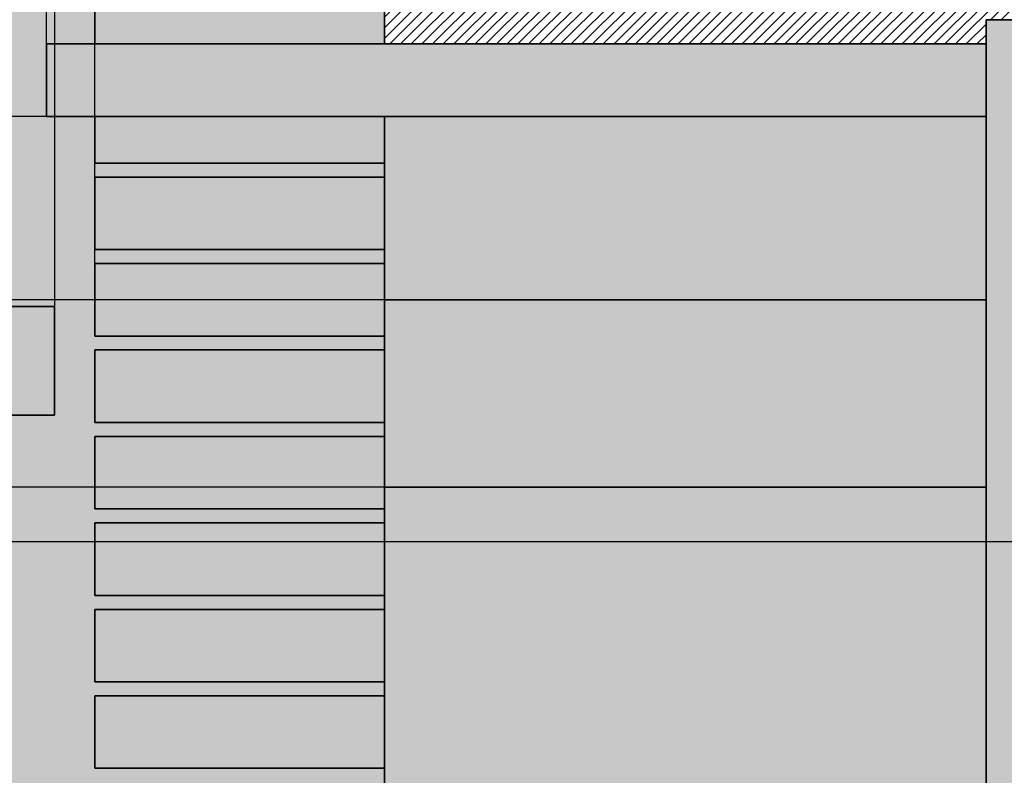
# Model space of a CAD drawing. Units: inches. Extents: x 126 to 726, y 86 to 888.
# Tile 10 of 13: x 426 to 589, y 486 to 611. Entities that reach past the tile are written whole.
import ezdxf

# ---------------------------------------------------------------- set-up
doc = ezdxf.new("R2010")
doc.units = ezdxf.units.IN
doc.header["$MEASUREMENT"] = 0
for name, color, linetype, lineweight in [('A-ANNO-DIMS', 2, 'Continuous', 18), ('A-ELEV', 7, 'Continuous', 35), ('A-ELEV-PATT', 8, 'Continuous', 13)]:
    doc.layers.add(name, color=color, linetype=linetype, lineweight=lineweight)
doc.styles.get("Standard").update_dxf_attribs({"font": 'arial.ttf'})
doc.dimstyles.get("Standard").update_dxf_attribs({"dimtxt": 6, "dimasz": 3, "dimexe": 0.18, "dimexo": 0.0625, "dimgap": 0.09, "dimtad": 0, "dimtih": 1, "dimtoh": 1, "dimdec": 0, "dimzin": 0, "dimdsep": 46, "dimlunit": 3, "dimtxsty": 'Standard', "dimcen": 0.09, "dimadec": 0, "dimazin": 0, "dimtfac": 1, "dimtdec": 0, "dimtofl": 0, "dimtmove": 0, "dimatfit": 3, "dimfxl": 1, "dimtolj": 1, "dimtzin": 0, "dimarcsym": 0})

# ---------------------------------------------------------------- blocks, each defined once
blk = doc.blocks.new('FACADE-STRIP')
for p, q in [((0, 0), (0, 12)), ((0, 12), (48, 12)), ((0, 0), (48, 0))]:
    blk.add_line(p, q)
blk = doc.blocks.new('*D13')
at = {"layer": 'A-ANNO-DIMS', "color": 0, "lineweight": -2, "transparency": 16777216}
for p, q in [((665.97, 642.98), (665.97, 90.21)), ((185.97, 126.98), (185.97, 90.21)), ((188.97, 90.39), (419.15, 90.39)), ((662.97, 90.39), (432.8, 90.39))]:
    blk.add_line(p, q, dxfattribs=at)
at = {"layer": 'A-ANNO-DIMS', "color": 0, "transparency": 16777216}
for points in [[(188.97, 90.89), (188.97, 89.89), (185.97, 90.39)], [(662.97, 90.89), (662.97, 89.89), (665.97, 90.39)]]:
    blk.add_solid(points, dxfattribs=at)
at = {"layer": 'Defpoints', "color": 0, "transparency": 16777216}
for p in [(665.97, 643.04), (185.97, 127.04), (665.97, 90.39)]:
    blk.add_point(p, dxfattribs=at)
at = {"layer": 'A-ANNO-DIMS', "color": 0, "transparency": 16777216, "insert": (425.97, 90.39), "char_height": 6, "attachment_point": 5}
blk.add_mtext('\\A1;480', dxfattribs=at)
blk = doc.blocks.new('*D21')
at = {"layer": 'A-ANNO-DIMS', "color": 0, "lineweight": -2, "transparency": 16777216}
for p, q in [((431.28, 563.58), (149.14, 563.58)), ((149.32, 560.58), (149.32, 557.74)), ((149.32, 548.58), (149.32, 551.43)), ((233.91, 545.58), (149.14, 545.58))]:
    blk.add_line(p, q, dxfattribs=at)
at = {"layer": 'A-ANNO-DIMS', "color": 0, "transparency": 16777216}
for points in [[(148.82, 560.58), (149.82, 560.58), (149.32, 563.58)], [(148.82, 548.58), (149.82, 548.58), (149.32, 545.58)]]:
    blk.add_solid(points, dxfattribs=at)
at = {"layer": 'Defpoints', "color": 0, "transparency": 16777216}
for p in [(149.32, 563.58), (431.34, 563.58), (233.97, 545.58)]:
    blk.add_point(p, dxfattribs=at)
at = {"layer": 'A-ANNO-DIMS', "color": 0, "transparency": 16777216, "insert": (149.32, 554.58), "char_height": 6, "attachment_point": 5}
blk.add_mtext('\\A1;18', dxfattribs=at)
blk = doc.blocks.new('*D22')
at = {"layer": 'A-ANNO-DIMS', "color": 0, "lineweight": -2, "transparency": 16777216}
for p, q in [((185.91, 847.04), (149.14, 847.04)), ((149.32, 844.04), (149.32, 708.47)), ((149.32, 566.58), (149.32, 702.16)), ((431.28, 563.58), (149.14, 563.58))]:
    blk.add_line(p, q, dxfattribs=at)
at = {"layer": 'A-ANNO-DIMS', "color": 0, "transparency": 16777216}
for points in [[(148.82, 844.04), (149.82, 844.04), (149.32, 847.04)], [(148.82, 566.58), (149.82, 566.58), (149.32, 563.58)]]:
    blk.add_solid(points, dxfattribs=at)
at = {"layer": 'Defpoints', "color": 0, "transparency": 16777216}
for p in [(149.32, 847.04), (185.97, 847.04), (431.34, 563.58)]:
    blk.add_point(p, dxfattribs=at)
at = {"layer": 'A-ANNO-DIMS', "color": 0, "transparency": 16777216, "insert": (149.32, 705.31), "char_height": 6, "attachment_point": 5}
blk.add_mtext('\\A1;283.46', dxfattribs=at)
blk = doc.blocks.new('*D34')
at = {"layer": 'A-ANNO-DIMS', "color": 0, "lineweight": -2, "transparency": 16777216}
for p, q in [((362.73, 524.68), (702.8, 524.68)), ((702.62, 521.68), (702.62, 482.84)), ((702.62, 437.68), (702.62, 476.53)), ((362.73, 434.68), (702.8, 434.68))]:
    blk.add_line(p, q, dxfattribs=at)
at = {"layer": 'A-ANNO-DIMS', "color": 0, "transparency": 16777216}
for points in [[(702.12, 521.68), (703.12, 521.68), (702.62, 524.68)], [(702.12, 437.68), (703.12, 437.68), (702.62, 434.68)]]:
    blk.add_solid(points, dxfattribs=at)
at = {"layer": 'Defpoints', "color": 0, "transparency": 16777216}
for p in [(362.67, 524.68), (702.62, 524.68), (362.67, 434.68)]:
    blk.add_point(p, dxfattribs=at)
at = {"layer": 'A-ANNO-DIMS', "color": 0, "transparency": 16777216, "insert": (702.62, 479.68), "char_height": 6, "attachment_point": 5}
blk.add_mtext('\\A1;90', dxfattribs=at)
blk = doc.blocks.new('*D41')
at = {"layer": 'A-ANNO-DIMS', "color": 0, "lineweight": -2, "transparency": 16777216}
for p, q in [((429.97, 607.1), (429.97, 883.87)), ((432.97, 883.69), (541.21, 883.69)), ((662.97, 883.69), (554.74, 883.69)), ((665.97, 607.1), (665.97, 883.87))]:
    blk.add_line(p, q, dxfattribs=at)
at = {"layer": 'A-ANNO-DIMS', "color": 0, "transparency": 16777216}
for points in [[(432.97, 884.19), (432.97, 883.19), (429.97, 883.69)], [(662.97, 884.19), (662.97, 883.19), (665.97, 883.69)]]:
    blk.add_solid(points, dxfattribs=at)
at = {"layer": 'Defpoints', "color": 0, "transparency": 16777216}
for p in [(665.97, 883.69), (429.97, 607.04), (665.97, 607.04)]:
    blk.add_point(p, dxfattribs=at)
at = {"layer": 'A-ANNO-DIMS', "color": 0, "transparency": 16777216, "insert": (547.97, 883.69), "char_height": 6, "attachment_point": 5}
blk.add_mtext('\\A1;236', dxfattribs=at)
blk = doc.blocks.new('*D43')
at = {"layer": 'A-ANNO-DIMS', "color": 0, "lineweight": -2, "transparency": 16777216}
for p, q in [((429.97, 595.1), (429.97, 883.87)), ((432.97, 883.69), (434.97, 883.69)), ((437.97, 585.06), (437.97, 883.87)), ((437.97, 883.69), (440.97, 883.69))]:
    blk.add_line(p, q, dxfattribs=at)
at = {"layer": 'A-ANNO-DIMS', "color": 0, "transparency": 16777216}
for points in [[(432.97, 884.19), (432.97, 883.19), (429.97, 883.69)], [(434.97, 884.19), (434.97, 883.19), (437.97, 883.69)]]:
    blk.add_solid(points, dxfattribs=at)
at = {"layer": 'Defpoints', "color": 0, "transparency": 16777216}
for p in [(437.97, 883.69), (429.97, 595.04), (437.97, 585)]:
    blk.add_point(p, dxfattribs=at)
at = {"layer": 'A-ANNO-DIMS', "color": 0, "transparency": 16777216, "insert": (443.04, 883.69), "char_height": 6, "attachment_point": 5}
blk.add_mtext('\\A1;8', dxfattribs=at)
blk = doc.blocks.new('*D44')
at = {"layer": 'A-ANNO-DIMS', "color": 0, "lineweight": -2, "transparency": 16777216}
for p, q in [((431.34, 563.65), (431.34, 883.87)), ((434.34, 883.69), (434.97, 883.69)), ((437.97, 570.75), (437.97, 883.87)), ((437.97, 883.69), (440.97, 883.69))]:
    blk.add_line(p, q, dxfattribs=at)
at = {"layer": 'A-ANNO-DIMS', "color": 0, "transparency": 16777216}
for points in [[(434.34, 884.19), (434.34, 883.19), (431.34, 883.69)], [(434.97, 884.19), (434.97, 883.19), (437.97, 883.69)]]:
    blk.add_solid(points, dxfattribs=at)
at = {"layer": 'Defpoints', "color": 0, "transparency": 16777216}
for p in [(437.97, 883.69), (437.97, 570.69), (431.34, 563.58)]:
    blk.add_point(p, dxfattribs=at)
at = {"layer": 'A-ANNO-DIMS', "color": 0, "transparency": 16777216, "insert": (451.2, 883.69), "char_height": 6, "attachment_point": 5}
blk.add_mtext('\\A1;6.636', dxfattribs=at)
blk = doc.blocks.new('*D58')
at = {"layer": 'A-ANNO-DIMS', "color": 0, "lineweight": -2, "transparency": 16777216}
for p, q in [((485.91, 533.68), (149.14, 533.68)), ((149.32, 530.68), (149.32, 453.52)), ((149.32, 370.04), (149.32, 447.21)), ((485.91, 367.04), (149.14, 367.04))]:
    blk.add_line(p, q, dxfattribs=at)
at = {"layer": 'A-ANNO-DIMS', "color": 0, "transparency": 16777216}
for points in [[(148.82, 530.68), (149.82, 530.68), (149.32, 533.68)], [(148.82, 370.04), (149.82, 370.04), (149.32, 367.04)]]:
    blk.add_solid(points, dxfattribs=at)
at = {"layer": 'Defpoints', "color": 0, "transparency": 16777216}
for p in [(149.32, 533.68), (485.97, 533.68), (485.97, 367.04)]:
    blk.add_point(p, dxfattribs=at)
at = {"layer": 'A-ANNO-DIMS', "color": 0, "transparency": 16777216, "insert": (149.32, 450.36), "char_height": 6, "attachment_point": 5}
blk.add_mtext('\\A1;166.64', dxfattribs=at)
blk = doc.blocks.new('*D59')
at = {"layer": 'A-ANNO-DIMS', "color": 0, "lineweight": -2, "transparency": 16777216}
for p, q in [((485.91, 564.68), (149.14, 564.68)), ((149.32, 561.68), (149.32, 552.34)), ((149.32, 536.68), (149.32, 546.03)), ((485.91, 533.68), (149.14, 533.68))]:
    blk.add_line(p, q, dxfattribs=at)
at = {"layer": 'A-ANNO-DIMS', "color": 0, "transparency": 16777216}
for points in [[(148.82, 561.68), (149.82, 561.68), (149.32, 564.68)], [(148.82, 536.68), (149.82, 536.68), (149.32, 533.68)]]:
    blk.add_solid(points, dxfattribs=at)
at = {"layer": 'Defpoints', "color": 0, "transparency": 16777216}
for p in [(149.32, 564.68), (485.97, 564.68), (485.97, 533.68)]:
    blk.add_point(p, dxfattribs=at)
at = {"layer": 'A-ANNO-DIMS', "color": 0, "transparency": 16777216, "insert": (149.32, 549.18), "char_height": 6, "attachment_point": 5}
blk.add_mtext('\\A1;31', dxfattribs=at)
blk = doc.blocks.new('*D60')
at = {"layer": 'A-ANNO-DIMS', "color": 0, "lineweight": -2, "transparency": 16777216}
for p, q in [((485.91, 595.04), (149.14, 595.04)), ((149.32, 592.04), (149.32, 583.02)), ((149.32, 567.68), (149.32, 576.71)), ((485.91, 564.68), (149.14, 564.68))]:
    blk.add_line(p, q, dxfattribs=at)
at = {"layer": 'A-ANNO-DIMS', "color": 0, "transparency": 16777216}
for points in [[(148.82, 592.04), (149.82, 592.04), (149.32, 595.04)], [(148.82, 567.68), (149.82, 567.68), (149.32, 564.68)]]:
    blk.add_solid(points, dxfattribs=at)
at = {"layer": 'Defpoints', "color": 0, "transparency": 16777216}
for p in [(149.32, 595.04), (485.97, 595.04), (485.97, 564.68)]:
    blk.add_point(p, dxfattribs=at)
at = {"layer": 'A-ANNO-DIMS', "color": 0, "transparency": 16777216, "insert": (149.32, 579.86), "char_height": 6, "attachment_point": 5}
blk.add_mtext('\\A1;30.36', dxfattribs=at)

msp = doc.modelspace()

# ---------------------------------------------------------------- hatches: boundary and pattern name
at = {"layer": 'A-ELEV-PATT'}
h = msp.add_hatch(color=256, dxfattribs=at)
h.dxf.hatch_style = 1
h.paths.add_polyline_path([(233.9749, 545.5846), (431.3386, 545.5846), (431.3386, 563.5846), (185.9749, 563.5846), (185.9749, 395.5846), (431.3386, 395.5846), (431.3386, 413.5846), (233.9749, 413.5846)])
h.paths.add_polyline_path([(233.9749, 835.0424), (485.9749, 835.0424), (605.9749, 835.0424), (605.9749, 847.0424), (485.9749, 847.0424), (185.9749, 847.0424), (185.9749, 606.5846), (233.9749, 606.5846)])
h.paths.add_polyline_path([(233.9749, 597.5846), (185.9749, 597.5846), (185.9749, 585.5846), (233.9749, 585.5846)])
h.paths.add_polyline_path([(233.9749, 580.5846), (185.9749, 580.5846), (185.9749, 568.5846), (233.9749, 568.5846)])
h = msp.add_hatch(color=256, dxfattribs=at)
h.dxf.hatch_style = 1
h.paths.add_polyline_path([(437.9749, 499.1312), (485.9749, 499.1312), (485.9749, 501.4423), (437.9749, 501.4423), (437.9749, 513.4423), (485.9749, 513.4423), (485.9749, 515.7534), (437.9749, 515.7534), (437.9749, 527.7534), (485.9749, 527.7534), (485.9749, 530.0646), (437.9749, 530.0646), (437.9749, 542.0646), (485.9749, 542.0646), (485.9749, 544.3757), (437.9749, 544.3757), (437.9749, 556.3757), (485.9749, 556.3757), (485.9749, 558.6868), (437.9749, 558.6868), (437.9749, 570.6868), (485.9749, 570.6868), (485.9749, 572.9979), (437.9749, 572.9979), (437.9749, 584.9979), (485.9749, 584.9979), (485.9749, 587.309), (437.9749, 587.309), (437.9749, 595.0424), (429.9749, 595.0424), (429.9749, 607.0424), (437.9749, 607.0424), (437.9749, 615.9312), (437.9749, 630.2423), (437.9749, 642.2423), (485.9749, 642.2423), (485.9749, 644.5534), (437.9749, 644.5534), (437.9749, 656.5534), (485.9749, 656.5534), (485.9749, 658.8645), (437.9749, 658.8645), (437.9749, 670.8645), (485.9749, 670.8645), (485.9749, 673.1757), (437.9749, 673.1757), (437.9749, 685.1757), (485.9749, 685.1757), (485.9749, 687.4868), (437.9749, 687.4868), (437.9749, 699.4868), (485.9749, 699.4868), (485.9749, 701.7979), (437.9749, 701.7979), (437.9749, 713.7979), (485.9749, 713.7979), (485.9749, 716.109), (437.9749, 716.109), (437.9749, 728.109), (485.9749, 728.109), (485.9749, 730.4201), (437.9749, 730.4201), (437.9749, 742.4201), (485.9749, 742.4201), (485.9749, 744.7312), (437.9749, 744.7312), (437.9749, 756.7312), (485.9749, 756.7312), (485.9749, 759.0423), (437.9749, 759.0423), (437.9749, 771.0423), (485.9749, 771.0423), (485.9749, 773.3534), (437.9749, 773.3534), (437.9749, 785.3534), (485.9749, 785.3534), (485.9749, 787.6645), (437.9749, 787.6645), (437.9749, 799.6645), (485.9749, 799.6645), (485.9749, 801.9756), (437.9749, 801.9756), (437.9749, 811.2868), (485.9749, 811.2868), (485.9749, 813.9756), (437.9749, 813.9756), (437.9749, 825.9756), (485.9749, 825.9756), (485.9749, 835.0424), (233.9749, 835.0424), (233.9749, 606.5846), (185.9749, 606.5846), (185.9749, 597.5846), (233.9749, 597.5846), (233.9749, 585.5846), (185.9749, 585.5846), (185.9749, 580.5846), (233.9749, 580.5846), (233.9749, 568.5846), (185.9749, 568.5846), (185.9749, 563.5846), (431.3386, 563.5846), (431.3386, 545.5846), (233.9749, 545.5846), (233.9749, 413.5846), (431.3386, 413.5846), (431.3386, 395.5846), (185.9749, 395.5846), (185.9749, 386.5846), (233.9749, 386.5846), (233.9749, 374.5846), (185.9749, 374.5846), (185.9749, 369.5846), (233.9749, 369.5846), (233.9749, 357.5846), (185.9749, 357.5846), (185.9749, 352.5846), (233.9749, 352.5846), (233.9749, 340.5846), (185.9749, 340.5846), (185.9749, 331.5846), (233.9749, 331.5846), (233.9749, 127.0424), (485.9749, 127.0424), (485.9749, 129.3535), (437.9749, 129.3535), (437.9749, 141.3535), (485.9749, 141.3535), (485.9749, 143.6646), (437.9749, 143.6646), (437.9749, 155.6646), (485.9749, 155.6646), (485.9749, 157.9757), (437.9749, 157.9757), (437.9749, 169.9757), (485.9749, 169.9757), (485.9749, 172.2868), (437.9749, 172.2868), (437.9749, 184.2868), (485.9749, 184.2868), (485.9749, 186.5979), (437.9749, 186.5979), (437.9749, 198.5979), (485.9749, 198.5979), (485.9749, 200.909), (437.9749, 200.909), (437.9749, 212.909), (485.9749, 212.909), (485.9749, 215.2201), (437.9749, 215.2201), (437.9749, 227.2201), (485.9749, 227.2201), (485.9749, 229.5312), (437.9749, 229.5312), (437.9749, 241.5312), (485.9749, 241.5312), (485.9749, 243.8424), (437.9749, 243.8424), (437.9749, 255.8424), (485.9749, 255.8424), (485.9749, 258.1535), (437.9749, 258.1535), (437.9749, 270.1535), (485.9749, 270.1535), (485.9749, 272.4646), (437.9749, 272.4646), (437.9749, 284.4646), (485.9749, 284.4646), (485.9749, 286.7757), (437.9749, 286.7757), (437.9749, 298.7757), (485.9749, 298.7757), (485.9749, 301.0868), (437.9749, 301.0868), (437.9749, 313.0868), (485.9749, 313.0868), (485.9749, 315.3979), (437.9749, 315.3979), (437.9749, 327.3979), (485.9749, 327.3979), (485.9749, 329.709), (437.9749, 329.709), (437.9749, 341.709), (485.9749, 341.709), (485.9749, 344.0201), (437.9749, 344.0201), (437.9749, 355.0424), (429.9749, 355.0424), (429.9749, 367.0424), (437.9749, 367.0424), (437.9749, 372.6423), (437.9749, 386.9535), (437.9749, 401.2646), (437.9749, 413.2646), (485.9749, 413.2646), (485.9749, 415.5757), (437.9749, 415.5757), (437.9749, 427.5757), (485.9749, 427.5757), (485.9749, 429.8868), (437.9749, 429.8868), (437.9749, 441.8868), (485.9749, 441.8868), (485.9749, 444.1979), (437.9749, 444.1979), (437.9749, 456.1979), (485.9749, 456.1979), (485.9749, 458.509), (437.9749, 458.509), (437.9749, 470.509), (485.9749, 470.509), (485.9749, 472.8201), (437.9749, 472.8201), (437.9749, 484.8201), (485.9749, 484.8201), (485.9749, 487.1312), (437.9749, 487.1312)])
h.paths.add_polyline_path([(299.6658, 533.6845), (371.6658, 533.6845), (371.6658, 425.6845), (299.6658, 425.6845)], flags=16)
h.paths.add_polyline_path([(308.6658, 524.6845), (362.6658, 524.6845), (362.6658, 434.6845), (308.6658, 434.6845)], flags=0)
h.paths.add_polyline_path([(317.7956, 603.3211, -0.4129833), (306.8418, 614.321, -0.94403766), (328.769, 615.5845, -0.04423165), (330.7031, 615.4048, -0.89973713), (352.5798, 615.6161, -0.4129833), (363.5336, 604.6162, -0.94403766), (341.6064, 603.3528, -0.04423165), (339.6723, 603.5324, -0.89973713)], flags=16)
h.paths.add_polyline_path([(319.7228, 604.5846, -0.02633223), (319.7726, 605.5306, -0.47905713), (308.8418, 614.321, -1), (326.8418, 614.321, -0.02633223), (326.7919, 613.375, -0.17413188), (332.826, 612.5948, -0.04918553), (332.6526, 614.3527, -1), (350.6526, 614.3527, -0.02633223), (350.6028, 613.4067, -0.47905713), (361.5336, 604.6162, -1), (343.5336, 604.6162, -0.02633223), (343.5834, 605.5622, -0.17413188), (337.5494, 606.3424, -0.04918553), (337.7228, 604.5846, -1)], flags=0)
h.paths.add_polyline_path([(328.769, 355.6561, -0.04423165), (330.7031, 355.4765, -0.89973713), (352.5798, 355.6878, -0.4129833), (363.5336, 344.6879, -0.94403766), (341.6064, 343.4244, -0.04423165), (339.6723, 343.604, -0.89973713), (317.7956, 343.3927, -0.4129833), (306.8418, 354.3926, -0.94403766)], flags=16)
h.paths.add_polyline_path([(326.8418, 354.3926, -0.02633223), (326.7919, 353.4466, -0.17413188), (332.826, 352.6664, -0.04918553), (332.6526, 354.4243, -1), (350.6526, 354.4243, -0.02633223), (350.6028, 353.4783, -0.47905713), (361.5336, 344.6879, -1), (343.5336, 344.6879, -0.02633223), (343.5834, 345.6339, -0.17413188), (337.5494, 346.4141, -0.04918553), (337.7228, 344.6562, -1), (319.7228, 344.6562, -0.02633223), (319.7726, 345.6022, -0.47905713), (308.8418, 354.3926, -1)], flags=0)
h.paths.add_polyline_path([(299.3189, 655.3527), (299.3189, 763.3527), (371.3189, 763.3527), (371.3189, 655.3527)], flags=16)
h.paths.add_polyline_path([(308.3189, 664.3527), (308.3189, 754.3527), (362.3189, 754.3527), (362.3189, 664.3527)], flags=0)
h.paths.add_polyline_path([(299.6658, 303.5875), (371.6658, 303.5875), (371.6658, 195.5875), (299.6658, 195.5875)], flags=16)
h.paths.add_polyline_path([(308.6658, 294.5875), (362.6658, 294.5875), (362.6658, 204.5875), (308.6658, 204.5875)], flags=0)
h.paths.add_polyline_path([(326.3038, 177.3867), (346.055, 177.3867, -0.41421356), (349.055, 174.3867), (349.055, 171.2378), (363.489, 171.2378, -0.41421356), (366.489, 168.2378), (366.489, 159.7133, -0.41421356), (363.489, 156.7133), (343.7379, 156.7133, -0.41421356), (340.7379, 159.7133), (340.7379, 162.8622), (330.5504, 162.8622), (330.5504, 159.7133, -0.41421356), (327.5504, 156.7133), (307.7992, 156.7133, -0.41421356), (304.7992, 159.7133), (304.7992, 168.2378, -0.41421356), (307.7992, 171.2378), (323.3038, 171.2378), (323.3038, 174.3867, -0.41421356)], flags=16)
h.paths.add_polyline_path([(326.3038, 175.3867), (346.055, 175.3867, -0.41421356), (347.055, 174.3867), (347.055, 169.2378), (363.489, 169.2378, -0.41421356), (364.489, 168.2378), (364.489, 159.7133, -0.41421356), (363.489, 158.7133), (343.7379, 158.7133, -0.41421356), (342.7379, 159.7133), (342.7379, 164.8622), (328.5504, 164.8622), (328.5504, 159.7133, -0.41421356), (327.5504, 158.7133), (307.7992, 158.7133, -0.41421356), (306.7992, 159.7133), (306.7992, 168.2378, -0.41421356), (307.7992, 169.2378), (325.3038, 169.2378), (325.3038, 174.3867, -0.41421356)], flags=0)
h = msp.add_hatch(dxfattribs=at)
h.set_pattern_fill('GRAVEL', color=256, scale=40)
h.paths.add_polyline_path([(437.9749, 642.2423), (485.9749, 642.2423), (485.9749, 644.5534), (437.9749, 644.5534), (437.9749, 656.5534), (485.9749, 656.5534), (485.9749, 658.8645), (437.9749, 658.8645), (437.9749, 670.8645), (485.9749, 670.8645), (485.9749, 673.1757), (437.9749, 673.1757), (437.9749, 685.1757), (485.9749, 685.1757), (485.9749, 687.4868), (437.9749, 687.4868), (437.9749, 699.4868), (485.9749, 699.4868), (485.9749, 701.7979), (437.9749, 701.7979), (437.9749, 713.7979), (485.9749, 713.7979), (485.9749, 716.109), (437.9749, 716.109), (437.9749, 728.109), (485.9749, 728.109), (485.9749, 730.4201), (437.9749, 730.4201), (437.9749, 742.4201), (485.9749, 742.4201), (485.9749, 744.7312), (437.9749, 744.7312), (437.9749, 756.7312), (485.9749, 756.7312), (485.9749, 759.0423), (437.9749, 759.0423), (437.9749, 771.0423), (485.9749, 771.0423), (485.9749, 773.3534), (437.9749, 773.3534), (437.9749, 785.3534), (485.9749, 785.3534), (485.9749, 787.6645), (437.9749, 787.6645), (437.9749, 799.6645), (485.9749, 799.6645), (485.9749, 801.9756), (437.9749, 801.9756), (437.9749, 811.2868), (485.9749, 811.2868), (485.9749, 813.9756), (437.9749, 813.9756), (437.9749, 825.9756), (485.9749, 825.9756), (485.9749, 835.0424), (233.9749, 835.0424), (233.9749, 606.5846), (185.9749, 606.5846), (185.9749, 597.5846), (233.9749, 597.5846), (233.9749, 585.5846), (185.9749, 585.5846), (185.9749, 580.5846), (233.9749, 580.5846), (233.9749, 568.5846), (185.9749, 568.5846), (185.9749, 563.5846), (431.3386, 563.5846), (431.3386, 545.5846), (233.9749, 545.5846), (233.9749, 413.5846), (431.3386, 413.5846), (431.3386, 395.5846), (185.9749, 395.5846), (185.9749, 386.5846), (233.9749, 386.5846), (233.9749, 374.5846), (185.9749, 374.5846), (185.9749, 369.5846), (233.9749, 369.5846), (233.9749, 357.5846), (185.9749, 357.5846), (185.9749, 352.5846), (233.9749, 352.5846), (233.9749, 340.5846), (185.9749, 340.5846), (185.9749, 331.5846), (233.9749, 331.5846), (233.9749, 127.0424), (485.9749, 127.0424), (485.9749, 129.3535), (437.9749, 129.3535), (437.9749, 141.3535), (485.9749, 141.3535), (485.9749, 143.6646), (437.9749, 143.6646), (437.9749, 155.6646), (485.9749, 155.6646), (485.9749, 157.9757), (437.9749, 157.9757), (437.9749, 169.9757), (485.9749, 169.9757), (485.9749, 172.2868), (437.9749, 172.2868), (437.9749, 184.2868), (485.9749, 184.2868), (485.9749, 186.5979), (437.9749, 186.5979), (437.9749, 198.5979), (485.9749, 198.5979), (485.9749, 200.909), (437.9749, 200.909), (437.9749, 212.909), (485.9749, 212.909), (485.9749, 215.2201), (437.9749, 215.2201), (437.9749, 227.2201), (485.9749, 227.2201), (485.9749, 229.5312), (437.9749, 229.5312), (437.9749, 241.5312), (485.9749, 241.5312), (485.9749, 243.8424), (437.9749, 243.8424), (437.9749, 255.8424), (485.9749, 255.8424), (485.9749, 258.1535), (437.9749, 258.1535), (437.9749, 270.1535), (485.9749, 270.1535), (485.9749, 272.4646), (437.9749, 272.4646), (437.9749, 284.4646), (485.9749, 284.4646), (485.9749, 286.7757), (437.9749, 286.7757), (437.9749, 298.7757), (485.9749, 298.7757), (485.9749, 301.0868), (437.9749, 301.0868), (437.9749, 313.0868), (485.9749, 313.0868), (485.9749, 315.3979), (437.9749, 315.3979), (437.9749, 327.3979), (485.9749, 327.3979), (485.9749, 329.709), (437.9749, 329.709), (437.9749, 341.709), (485.9749, 341.709), (485.9749, 344.0201), (437.9749, 344.0201), (437.9749, 355.0424), (429.9749, 355.0424), (429.9749, 367.0424), (437.9749, 367.0424), (437.9749, 372.6423), (437.9749, 386.9535), (437.9749, 401.2646), (437.9749, 413.2646), (485.9749, 413.2646), (485.9749, 415.5757), (437.9749, 415.5757), (437.9749, 427.5757), (485.9749, 427.5757), (485.9749, 429.8868), (437.9749, 429.8868), (437.9749, 441.8868), (485.9749, 441.8868), (485.9749, 444.1979), (437.9749, 444.1979), (437.9749, 456.1979), (485.9749, 456.1979), (485.9749, 458.509), (437.9749, 458.509), (437.9749, 470.509), (485.9749, 470.509), (485.9749, 472.8201), (437.9749, 472.8201), (437.9749, 484.8201), (485.9749, 484.8201), (485.9749, 487.1312), (437.9749, 487.1312), (437.9749, 499.1312), (485.9749, 499.1312), (485.9749, 501.4423), (437.9749, 501.4423), (437.9749, 513.4423), (485.9749, 513.4423), (485.9749, 515.7534), (437.9749, 515.7534), (437.9749, 527.7534), (485.9749, 527.7534), (485.9749, 530.0646), (437.9749, 530.0646), (437.9749, 542.0646), (485.9749, 542.0646), (485.9749, 544.3757), (437.9749, 544.3757), (437.9749, 556.3757), (485.9749, 556.3757), (485.9749, 558.6868), (437.9749, 558.6868), (437.9749, 570.6868), (485.9749, 570.6868), (485.9749, 572.9979), (437.9749, 572.9979), (437.9749, 584.9979), (485.9749, 584.9979), (485.9749, 587.309), (437.9749, 587.309), (437.9749, 595.0424), (429.9749, 595.0424), (429.9749, 607.0424), (437.9749, 607.0424), (437.9749, 615.9312), (437.9749, 630.2423)])
h.paths.add_polyline_path([(371.3189, 655.3527), (299.3189, 655.3527), (299.3189, 763.3527), (371.3189, 763.3527)], flags=16)
h.paths.add_polyline_path([(363.5336, 604.6162, -0.94403766), (341.6064, 603.3528, -0.04423165), (339.6723, 603.5324, -0.89973713), (317.7956, 603.3211, -0.4129833), (306.8418, 614.321, -0.94403766), (328.769, 615.5845, -0.04423165), (330.7031, 615.4048, -0.89973713), (352.5798, 615.6161, -0.4129833)], flags=16)
h.paths.add_polyline_path([(361.5336, 604.6162, -1), (343.5336, 604.6162, -0.02633223), (343.5834, 605.5622, -0.17413188), (337.5494, 606.3424, -0.04918553), (337.7228, 604.5846, -1), (319.7228, 604.5846, -0.02633223), (319.7726, 605.5306, -0.47905713), (308.8418, 614.321, -1), (326.8418, 614.321, -0.02633223), (326.7919, 613.375, -0.17413188), (332.826, 612.5948, -0.04918553), (332.6526, 614.3527, -1), (350.6526, 614.3527, -0.02633223), (350.6028, 613.4067, -0.47905713)], flags=0)
h.paths.add_polyline_path([(362.3189, 664.3527), (308.3189, 664.3527), (308.3189, 754.3527), (362.3189, 754.3527)], flags=0)
h.paths.add_polyline_path([(371.6658, 533.6845), (371.6658, 425.6845), (299.6658, 425.6845), (299.6658, 533.6845)], flags=16)
h.paths.add_polyline_path([(362.6658, 524.6845), (362.6658, 434.6845), (308.6658, 434.6845), (308.6658, 524.6845)], flags=0)
h.paths.add_polyline_path([(352.5798, 355.6878, -0.4129833), (363.5336, 344.6879, -0.94403766), (341.6064, 343.4244, -0.04423165), (339.6723, 343.604, -0.89973713), (317.7956, 343.3927, -0.4129833), (306.8418, 354.3926, -0.94403766), (328.769, 355.6561, -0.04423165), (330.7031, 355.4765, -0.89973713)], flags=16)
h.paths.add_polyline_path([(350.6526, 354.4243, -0.02633223), (350.6028, 353.4783, -0.47905713), (361.5336, 344.6879, -1), (343.5336, 344.6879, -0.02633223), (343.5834, 345.6339, -0.17413188), (337.5494, 346.4141, -0.04918553), (337.7228, 344.6562, -1), (319.7228, 344.6562, -0.02633223), (319.7726, 345.6022, -0.47905713), (308.8418, 354.3926, -1), (326.8418, 354.3926, -0.02633223), (326.7919, 353.4466, -0.17413188), (332.826, 352.6664, -0.04918553), (332.6526, 354.4243, -1)], flags=0)
h.paths.add_polyline_path([(371.6658, 303.5875), (371.6658, 195.5875), (299.6658, 195.5875), (299.6658, 303.5875)], flags=16)
h.paths.add_polyline_path([(362.6658, 294.5875), (362.6658, 204.5875), (308.6658, 204.5875), (308.6658, 294.5875)], flags=0)
h.paths.add_polyline_path([(346.055, 177.3867, -0.41421356), (349.055, 174.3867), (349.055, 171.2378), (363.489, 171.2378, -0.41421356), (366.489, 168.2378), (366.489, 159.7133, -0.41421356), (363.489, 156.7133), (343.7379, 156.7133, -0.41421356), (340.7379, 159.7133), (340.7379, 162.8622), (330.5504, 162.8622), (330.5504, 159.7133, -0.41421356), (327.5504, 156.7133), (307.7992, 156.7133, -0.41421356), (304.7992, 159.7133), (304.7992, 168.2378, -0.41421356), (307.7992, 171.2378), (323.3038, 171.2378), (323.3038, 174.3867, -0.41421356), (326.3038, 177.3867)], flags=16)
h.paths.add_polyline_path([(346.055, 175.3867, -0.41421356), (347.055, 174.3867), (347.055, 169.2378), (363.489, 169.2378, -0.41421356), (364.489, 168.2378), (364.489, 159.7133, -0.41421356), (363.489, 158.7133), (343.7379, 158.7133, -0.41421356), (342.7379, 159.7133), (342.7379, 164.8622), (328.5504, 164.8622), (328.5504, 159.7133, -0.41421356), (327.5504, 158.7133), (307.7992, 158.7133, -0.41421356), (306.7992, 159.7133), (306.7992, 168.2378, -0.41421356), (307.7992, 169.2378), (325.3038, 169.2378), (325.3038, 174.3867, -0.41421356), (326.3038, 175.3867)], flags=0)
h = msp.add_hatch(color=256, dxfattribs=at)
h.dxf.hatch_style = 1
h.paths.add_polyline_path([(485.9749, 427.5757), (437.9749, 427.5757), (437.9749, 415.5757), (485.9749, 415.5757)])
h.paths.add_polyline_path([(485.9749, 441.8868), (437.9749, 441.8868), (437.9749, 429.8868), (485.9749, 429.8868)])
h.paths.add_polyline_path([(485.9749, 456.1979), (437.9749, 456.1979), (437.9749, 444.1979), (485.9749, 444.1979)])
h.paths.add_polyline_path([(485.9749, 470.509), (437.9749, 470.509), (437.9749, 458.509), (485.9749, 458.509)])
h.paths.add_polyline_path([(485.9749, 484.8201), (437.9749, 484.8201), (437.9749, 472.8201), (485.9749, 472.8201)])
h.paths.add_polyline_path([(485.9749, 499.1312), (437.9749, 499.1312), (437.9749, 487.1312), (485.9749, 487.1312)])
h.paths.add_polyline_path([(485.9749, 513.4423), (437.9749, 513.4423), (437.9749, 501.4423), (485.9749, 501.4423)])
h.paths.add_polyline_path([(485.9749, 527.7534), (437.9749, 527.7534), (437.9749, 515.7534), (485.9749, 515.7534)])
h.paths.add_polyline_path([(485.9749, 542.0646), (437.9749, 542.0646), (437.9749, 530.0646), (485.9749, 530.0646)])
h.paths.add_polyline_path([(485.9749, 556.3757), (437.9749, 556.3757), (437.9749, 544.3757), (485.9749, 544.3757)])
h.paths.add_polyline_path([(485.9749, 570.6868), (437.9749, 570.6868), (437.9749, 558.6868), (485.9749, 558.6868)])
h.paths.add_polyline_path([(485.9749, 584.9979), (437.9749, 584.9979), (437.9749, 572.9979), (485.9749, 572.9979)])
h.paths.add_polyline_path([(485.9749, 595.0424), (437.9749, 595.0424), (437.9749, 587.309), (485.9749, 587.309)])
h.paths.add_polyline_path([(485.9749, 613.6201), (437.9749, 613.6201), (437.9749, 607.0424), (485.9749, 607.0424)])
h.paths.add_polyline_path([(485.9749, 627.9312), (437.9749, 627.9312), (437.9749, 615.9312), (485.9749, 615.9312)])
h.paths.add_polyline_path([(485.9749, 642.2423), (437.9749, 642.2423), (437.9749, 630.2423), (485.9749, 630.2423)])
h.paths.add_polyline_path([(485.9749, 656.5534), (437.9749, 656.5534), (437.9749, 644.5534), (485.9749, 644.5534)])
h.paths.add_polyline_path([(485.9749, 670.8645), (437.9749, 670.8645), (437.9749, 658.8645), (485.9749, 658.8645)])
h.paths.add_polyline_path([(485.9749, 685.1757), (437.9749, 685.1757), (437.9749, 673.1757), (485.9749, 673.1757)])
h.paths.add_polyline_path([(485.9749, 699.4868), (437.9749, 699.4868), (437.9749, 687.4868), (485.9749, 687.4868)])
h.paths.add_polyline_path([(485.9749, 713.7979), (437.9749, 713.7979), (437.9749, 701.7979), (485.9749, 701.7979)])
h.paths.add_polyline_path([(485.9749, 728.109), (437.9749, 728.109), (437.9749, 716.109), (485.9749, 716.109)])
h.paths.add_polyline_path([(485.9749, 742.4201), (437.9749, 742.4201), (437.9749, 730.4201), (485.9749, 730.4201)])
h.paths.add_polyline_path([(485.9749, 756.7312), (437.9749, 756.7312), (437.9749, 744.7312), (485.9749, 744.7312)])
h.paths.add_polyline_path([(485.9749, 771.0423), (437.9749, 771.0423), (437.9749, 759.0423), (485.9749, 759.0423)])
h.paths.add_polyline_path([(485.9749, 785.3534), (437.9749, 785.3534), (437.9749, 773.3534), (485.9749, 773.3534)])
h.paths.add_polyline_path([(485.9749, 799.6645), (437.9749, 799.6645), (437.9749, 787.6645), (485.9749, 787.6645)])
h.paths.add_polyline_path([(485.9749, 811.2868), (437.9749, 811.2868), (437.9749, 801.9756), (485.9749, 801.9756)])
h.paths.add_polyline_path([(485.9749, 825.9756), (437.9749, 825.9756), (437.9749, 813.9756), (485.9749, 813.9756)])
h = msp.add_hatch(dxfattribs=at)
h.set_pattern_fill('ANSI31', color=256, scale=10)
h.paths.add_polyline_path([(585.5818, 607.0424), (585.5818, 611.0424), (603.5818, 611.0424), (603.5818, 607.0424), (611.5818, 607.0424), (611.5818, 611.0424), (629.5818, 611.0424), (629.5818, 607.0424), (637.5818, 607.0424), (637.5818, 611.0424), (655.5818, 611.0424), (655.5818, 607.0424), (665.9749, 607.0424), (665.9749, 643.0424), (485.9749, 643.0424), (485.9749, 607.0424)])
h = msp.add_hatch(color=256, dxfattribs=at)
h.dxf.hatch_style = 1
h.paths.add_polyline_path([(655.5818, 607.0424), (655.5818, 611.0424), (637.5818, 611.0424), (637.5818, 355.0424), (655.5818, 355.0424)])
h.paths.add_polyline_path([(629.5818, 611.0424), (611.5818, 611.0424), (611.5818, 355.0424), (629.5818, 355.0424)])
h.paths.add_polyline_path([(585.5818, 355.0424), (603.5818, 355.0424), (603.5818, 611.0424), (585.5818, 611.0424), (585.5818, 607.0424)])
h = msp.add_hatch(color=256, dxfattribs=at)
h.dxf.hatch_style = 1
h.paths.add_polyline_path([(437.9749, 367.0424), (429.9749, 367.0424), (429.9749, 355.0424), (437.9749, 355.0424), (585.5818, 355.0424), (585.5818, 367.0424)])
h.paths.add_polyline_path([(585.5818, 595.0424), (585.5818, 607.0424), (437.9749, 607.0424), (429.9749, 607.0424), (429.9749, 595.0424), (437.9749, 595.0424)])
h = msp.add_hatch(color=256, dxfattribs=at)
h.dxf.hatch_style = 1
h.paths.add_polyline_path([(485.9749, 595.0424), (485.9749, 564.6845), (585.5818, 564.6845), (585.5818, 595.0424)])
h.paths.add_polyline_path([(660.0469, 325.0424), (660.0469, 355.0424), (485.9749, 355.0424), (485.9749, 325.0424)])
h = msp.add_hatch(color=256, dxfattribs=at)
h.dxf.hatch_style = 1
h.paths.add_polyline_path([(585.5818, 564.6845), (485.9749, 564.6845), (485.9749, 533.6845), (585.5818, 533.6845)])
h = msp.add_hatch(color=256, dxfattribs=at)
h.dxf.hatch_style = 1
h.paths.add_polyline_path([(585.5818, 533.6845), (485.9749, 533.6845), (485.9749, 403.0424), (585.5818, 403.0424)])
h.paths.add_polyline_path([(515.4403, 467.321), (515.4403, 463.4817), (501.8163, 463.4817), (501.8163, 467.321)], flags=16)

# ---------------------------------------------------------------- linework, layer by layer
at = {"layer": 'A-ELEV'}
for p, q in [((485.9749, 607.0424), (485.9749, 835.0424)), ((437.9749, 607.0424), (437.9749, 615.9312)), ((585.5818, 611.0424), (585.5818, 607.0424)), ((603.5818, 611.0424), (585.5818, 611.0424)), ((429.9749, 595.0424), (429.9749, 607.0424)), ((429.9749, 607.0424), (437.9749, 607.0424)), ((437.9749, 607.0424), (585.5818, 607.0424)), ((585.5818, 355.0424), (585.5818, 607.0424)), ((437.9749, 595.0424), (429.9749, 595.0424)), ((437.9749, 587.309), (437.9749, 595.0424)), ((585.5818, 595.0424), (437.9749, 595.0424)), ((485.9749, 367.0424), (485.9749, 595.0424)), ((437.9749, 587.309), (485.9749, 587.309)), ((485.9749, 564.6845), (585.5818, 564.6845)), ((431.3386, 563.5846), (185.9749, 563.5846)), ((431.3386, 545.5846), (431.3386, 563.5846)), ((431.3386, 545.5846), (233.9749, 545.5846)), ((485.9749, 533.6845), (585.5818, 533.6845))]:
    msp.add_line(p, q, dxfattribs=at)

# ---------------------------------------------------------------- block references
for p in [(437.975, 572.9974), (437.975, 558.6863), (437.975, 544.3752), (437.975, 530.0641), (437.975, 515.753), (437.975, 501.4419), (437.975, 487.1307)]:
    msp.add_blockref('FACADE-STRIP', p, dxfattribs=at)

# ---------------------------------------------------------------- dimensions: what is measured, and where the dimension line sits
at = {"layer": 'A-ANNO-DIMS'}
for base, p1, p2, override, picture, middle in [((665.9749, 883.6924), (429.9749, 607.0424), (665.9749, 607.0424), {"dimdec": 0, "dimlfac": 1, "dimrnd": 0, "dimzin": 0, "dimdsep": 46, "dimlunit": 2}, '*D41', (547.9749, 883.6924)), ((437.9749, 883.6924), (429.9749, 595.0424), (437.9749, 584.9979), {"dimdec": 0, "dimlfac": 1, "dimrnd": 0, "dimzin": 0, "dimdsep": 46, "dimlunit": 2}, '*D43', (443.0417, 883.6924)), ((437.9749, 883.6924), (431.3386, 563.5846), (437.9749, 570.6868), {"dimdec": 3, "dimlfac": 1, "dimrnd": 0, "dimzin": 0, "dimdsep": 46, "dimlunit": 2}, '*D44', (451.2027, 883.6924)), ((665.9749, 90.3924), (185.9749, 127.0424), (665.9749, 643.0424), {"dimdec": 0, "dimlfac": 1, "dimrnd": 0, "dimzin": 0, "dimdsep": 46, "dimlunit": 2}, '*D13', (425.9749, 90.3924))]:
    dim = msp.add_linear_dim(base=base, p1=p1, p2=p2, dimstyle='Standard', override=override, dxfattribs=at)
    dim.commit()
    dim.dimension.update_dxf_attribs({"geometry": picture, "text_midpoint": middle})
for base, p1, p2, override, picture, middle in [((149.3249, 847.0424), (431.3386, 563.5846), (185.9749, 847.0424), {"dimdec": 2, "dimlfac": 1, "dimrnd": 0, "dimzin": 0, "dimdsep": 46, "dimlunit": 2}, '*D22', (149.3249, 705.3135)), ((149.3249, 595.0424), (485.9749, 564.6845), (485.9749, 595.0424), {"dimdec": 2, "dimlfac": 1, "dimrnd": 0, "dimzin": 0, "dimdsep": 46, "dimlunit": 2}, '*D60', (149.3249, 579.8634)), ((149.3249, 564.6845), (485.9749, 533.6845), (485.9749, 564.6845), {"dimdec": 0, "dimlfac": 1, "dimrnd": 0, "dimzin": 0, "dimdsep": 46, "dimlunit": 2}, '*D59', (149.3249, 549.1845)), ((149.3249, 563.5846), (233.9749, 545.5846), (431.3386, 563.5846), {"dimdec": 0, "dimlfac": 1, "dimrnd": 0, "dimzin": 0, "dimdsep": 46, "dimlunit": 2}, '*D21', (149.3249, 554.5846)), ((149.3249, 533.6845), (485.9749, 367.0424), (485.9749, 533.6845), {"dimdec": 2, "dimlfac": 1, "dimrnd": 0, "dimzin": 0, "dimdsep": 46, "dimlunit": 2}, '*D58', (149.3249, 450.3634)), ((702.6249, 524.6845), (362.6658, 434.6845), (362.6658, 524.6845), {"dimdec": 0, "dimlfac": 1, "dimrnd": 0, "dimzin": 0, "dimdsep": 46, "dimlunit": 2}, '*D34', (702.6249, 479.6845))]:
    dim = msp.add_linear_dim(base=base, p1=p1, p2=p2, angle=90, dimstyle='Standard', override=override, dxfattribs=at)
    dim.commit()
    dim.dimension.update_dxf_attribs({"geometry": picture, "text_midpoint": middle})

doc.saveas('drawing.dxf')
